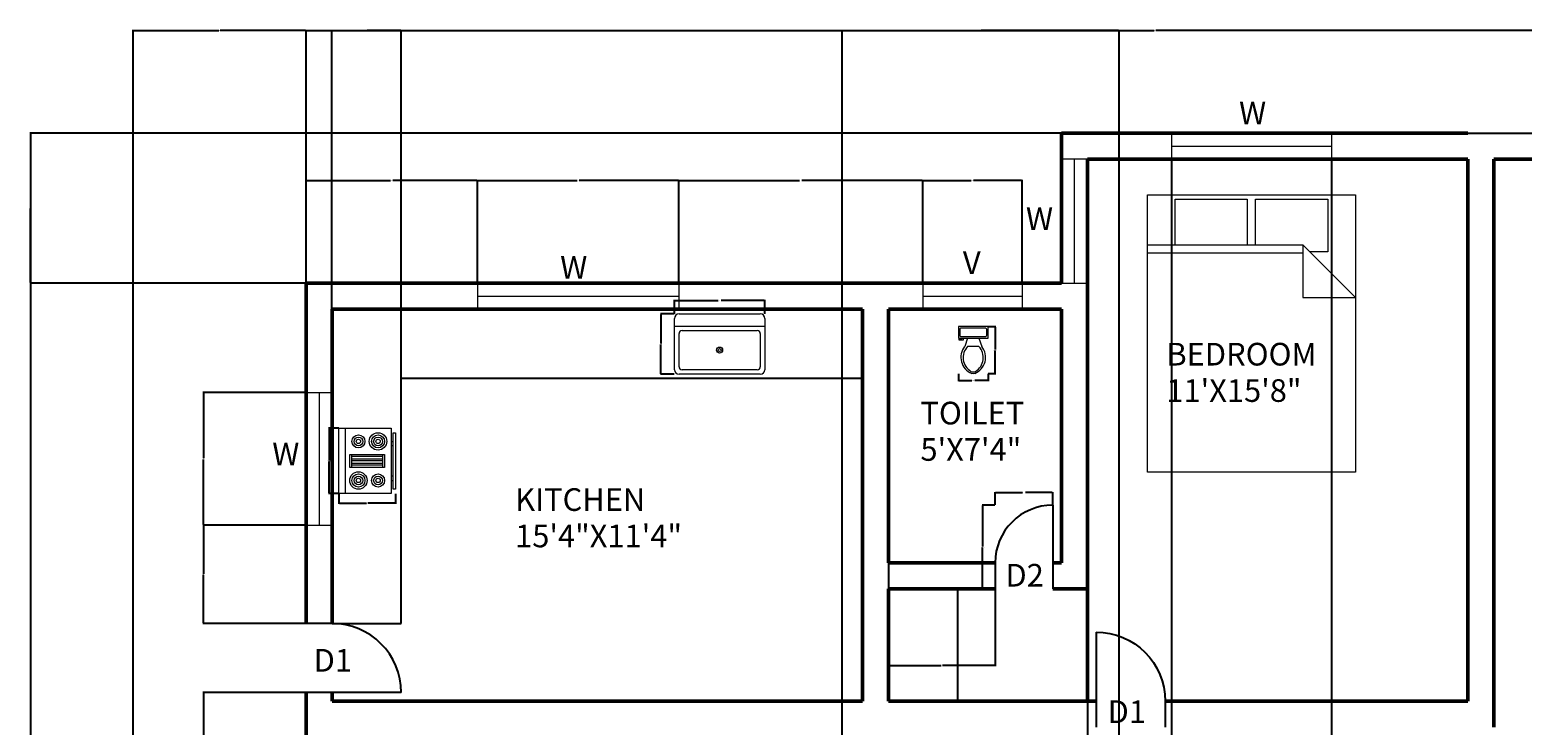
# Model space of a CAD drawing. Units: feet. Extents: x 1544 to 2324, y 1847 to 2475.
# Tile 3 of 4: x 1544 to 2061, y 2234 to 2475. Entities that reach past the tile are written whole.
import ezdxf

# ---------------------------------------------------------------- set-up
doc = ezdxf.new("R2010")
doc.units = ezdxf.units.FT
for name, color, linetype, lineweight in [('A-ANNO-DIMS', 2, 'Continuous', 18), ('A-ANNO-TEXT', 7, 'Continuous', 18), ('A-AREA-IDEN', 7, 'Continuous', 20), ('A-DOOR', 4, 'Continuous', 25), ('A-EQPM', 8, 'Continuous', 18), ('A-FLOR-CASE', 8, 'Continuous', 25), ('A-FLOR-FIXT', 9, 'Continuous', 18), ('A-FURN', 8, 'Continuous', 18), ('A-GLAZ', 4, 'Continuous', 18), ('A-WALL', 7, 'Continuous', 50), ('C-PROP', 3, 'Continuous', 25)]:
    doc.layers.add(name, color=color, linetype=linetype, lineweight=lineweight)
doc.styles.get("Standard").update_dxf_attribs({"font": 'arial.ttf'})
doc.dimstyles.get("Standard").update_dxf_attribs({"dimtxt": 0.18, "dimasz": 0.18, "dimexe": 0.18, "dimexo": 0.0625, "dimgap": 0.09, "dimtad": 0, "dimtih": 1, "dimtoh": 1, "dimdec": 4, "dimzin": 0, "dimdsep": 46, "dimtxsty": 'Standard', "dimcen": 0.09, "dimadec": 0, "dimazin": 0, "dimtfac": 1, "dimtdec": 4, "dimtofl": 0, "dimtmove": 0, "dimatfit": 3, "dimfxl": 1, "dimtolj": 1, "dimtzin": 0, "dimarcsym": 0})

# ---------------------------------------------------------------- blocks, each defined once
blk = doc.blocks.new('Sink-single - 30 in top')
blk.add_line((-15, -3.999996), (15, -3.999996))
for points in [[(-13.5, 0), (13.5, 0)], [(-15, -18.499996), (-15, -1.5)], [(15, -1.5), (15, -18.499996)], [(-13.5, -17.499996), (-13.5, -6.499996)], [(-12.5, -5.499996), (12.5, -5.499996)], [(13.5, -6.499996), (13.5, -17.499996)], [(12.5, -18.499996), (-12.5, -18.499996)], [(13.5, -19.999996), (-13.5, -19.999996)]]:
    blk.add_lwpolyline(points)
for radius in [1, 0.5]:
    blk.add_circle((0, -11.999996), radius)
for centre, radius, start, end in [((-13.5, -1.5), 1.5, 90, 180), ((13.5, -1.5), 1.5, 0, 90), ((-12.5, -6.499996), 1, 90, 180), ((12.5, -6.499996), 1, 0, 90), ((-13.5, -18.499996), 1.5, 180, 270), ((-12.5, -17.499996), 1, 180, 270), ((12.5, -17.499996), 1, 270, 0), ((13.5, -18.499996), 1.5, 270, 0)]:
    blk.add_arc(centre, radius, start, end)
blk = doc.blocks.new('Range-Oven - 30 in top')
for p, q in [((0, -3), (30, -3)), ((12, -6), (18, -6)), ((13, -20), (13, -6)), ((14, -6), (14, -20)), ((15, -20), (15, -6)), ((16, -6), (16, -20)), ((17, -20), (17, -6)), ((18, -20), (12, -20)), ((6, -24), (6, -25)), ((8, -25), (8, -24)), ((22, -25), (22, -24)), ((24, -24), (24, -25))]:
    blk.add_line(p, q)
for points in [[(0, -24), (0, 0), (30, 0), (30, -24)], [(12, -21), (12, -5), (18, -5), (18, -21)], [(2, -26), (2, -25), (28, -25), (28, -26)]]:
    blk.add_lwpolyline(points, close=True)
for centre, radius in [((6, -9), 4), ((6, -9), 3), ((24, -9), 3), ((6, -9), 2), ((6, -9), 1), ((24, -9), 2), ((24, -9), 1), ((6, -18), 3), ((6, -18), 2), ((6, -18), 1), ((24, -18), 4), ((24, -18), 3), ((24, -18), 2), ((24, -18), 1)]:
    blk.add_circle(centre, radius)
blk = doc.blocks.new('Toilet - top')
for p, q in [((-10, -8.5), (-8, -8.5)), ((-10, -9.5), (-10, -8.5)), ((-7, -9.5), (-10, -9.5)), ((-8, -8.5), (-8, -8)), ((-7, -8), (-7, -9.5)), ((-4, -8), (-6, -14)), ((4, -8), (6, -14)), ((9.5, -6), (9.5, -2)), ((4, -14), (-4, -14))]:
    blk.add_line(p, q)
blk.add_lwpolyline([(10.5, -8), (10.5, 0), (-10.5, 0), (-10.5, -8)], close=True)
for points in [[(-9.5, -2), (-9.5, -6)], [(8.5, -1), (-8.5, -1)], [(-8.5, -7), (8.5, -7)]]:
    blk.add_lwpolyline(points)
for centre, radius, start, end in [((-8.6, -1.9), 0.884, 81.8699, 188.1301), ((-8.6, -6.1), 0.884, 171.8699, 278.1301), ((8.6, -1.9), 0.884, 351.8699, 98.1301), ((8.6, -6.1), 0.884, 261.8699, 8.1301), ((3.5, -21.6), 12.2, 141.4691, 247.9714), ((4.2, -21.8), 11.3, 136.3677, 238.9468), ((-3.5, -21.6), 12.2, 292.0284, 38.5307), ((-4.2, -21.8), 11.3, 301.053, 43.6321), ((0, -27.9), 4, 245.7318, 294.2682), ((0, -29), 4, 254.8605, 285.1395)]:
    blk.add_arc(centre, radius, start, end)
blk = doc.blocks.new('Bed - Queen')
for p, q in [((0, -80.00003), (0, 0)), ((0, 0), (59.99999, 0)), ((59.99999, 0), (59.99999, -80.00003)), ((7.99999, -1.2), (28.79998, -1.2)), ((7.99999, -14.4), (7.99999, -1.2)), ((28.79998, -1.2), (28.79998, -14.4)), ((31.19999, -1.2), (51.99999, -1.2)), ((31.19999, -14.4), (31.19999, -1.2)), ((51.99999, -1.2), (51.99999, -16.4)), ((0, -14.4), (44.8, -14.4)), ((44.8, -16.8), (0, -16.8)), ((59.99999, -29.6), (44.8, -14.4)), ((44.8, -14.4), (44.8, -29.6)), ((51.99999, -16.4), (46.79936, -16.4)), ((44.8, -29.6), (59.99999, -29.6)), ((59.99999, -80.00003), (0, -80.00003))]:
    blk.add_line(p, q)
blk = doc.blocks.new('DOOR-SINGLE-R24')
for p, q in [((9, 24), (0, 24)), ((33, 0), (0, 0))]:
    blk.add_line(p, q)
blk.add_arc((9, 0), 24, 0, 90)
blk = doc.blocks.new('DOOR-SINGLE-R20')
for p, q in [((20, 29), (20, 0)), ((0, 9), (0, 0))]:
    blk.add_line(p, q)
blk.add_arc((20, 9), 20, 90, 180)
blk = doc.blocks.new('*D13')
at = {"layer": 'A-ANNO-DIMS', "color": 0, "lineweight": -2, "transparency": 16777216}
for p, q in [((1878.49, 2310.67), (1874.02, 2310.67)), ((1874.2, 2310.49), (1874.2, 2296.35)), ((1874.2, 2281.85), (1874.2, 2295.99)), ((1878.49, 2281.67), (1874.02, 2281.67))]:
    blk.add_line(p, q, dxfattribs=at)
at = {"layer": 'A-ANNO-DIMS', "color": 0, "transparency": 16777216}
for points in [[(1874.17, 2310.49), (1874.23, 2310.49), (1874.2, 2310.67)], [(1874.17, 2281.85), (1874.23, 2281.85), (1874.2, 2281.67)]]:
    blk.add_solid(points, dxfattribs=at)
at = {"layer": 'Defpoints', "color": 0, "transparency": 16777216}
for p in [(1874.2, 2310.67), (1878.55, 2310.67), (1878.55, 2281.67)]:
    blk.add_point(p, dxfattribs=at)
at = {"layer": 'A-ANNO-DIMS', "color": 0, "transparency": 16777216, "insert": (1874.2, 2296.17), "char_height": 0.18, "attachment_point": 5}
blk.add_mtext('\\A1;D2 29 TYP.', dxfattribs=at)
blk = doc.blocks.new('*D14')
at = {"layer": 'A-ANNO-DIMS', "color": 0, "lineweight": -2, "transparency": 16777216}
for p, q in [((1878.55, 2310.73), (1878.55, 2315.2)), ((1878.73, 2315.02), (1888.02, 2315.02)), ((1898.37, 2315.02), (1889.08, 2315.02)), ((1898.55, 2310.73), (1898.55, 2315.2))]:
    blk.add_line(p, q, dxfattribs=at)
at = {"layer": 'A-ANNO-DIMS', "color": 0, "transparency": 16777216}
for points in [[(1878.73, 2315.05), (1878.73, 2314.99), (1878.55, 2315.02)], [(1898.37, 2315.05), (1898.37, 2314.99), (1898.55, 2315.02)]]:
    blk.add_solid(points, dxfattribs=at)
at = {"layer": 'Defpoints', "color": 0, "transparency": 16777216}
for p in [(1898.55, 2315.02), (1878.55, 2310.67), (1898.55, 2310.67)]:
    blk.add_point(p, dxfattribs=at)
at = {"layer": 'A-ANNO-DIMS', "color": 0, "transparency": 16777216, "insert": (1888.55, 2315.02), "char_height": 0.18, "attachment_point": 5}
blk.add_mtext('\\A1;20 TYP.', dxfattribs=at)
blk = doc.blocks.new('*D15')
at = {"layer": 'A-ANNO-DIMS', "color": 0, "lineweight": -2, "transparency": 16777216}
for p, q in [((1876.19, 2372.55), (1878.75, 2372.55)), ((1878.57, 2372.37), (1878.57, 2364.6)), ((1878.57, 2356.47), (1878.57, 2364.24)), ((1876.19, 2356.29), (1878.75, 2356.29))]:
    blk.add_line(p, q, dxfattribs=at)
at = {"layer": 'A-ANNO-DIMS', "color": 0, "transparency": 16777216}
for points in [[(1878.54, 2372.37), (1878.6, 2372.37), (1878.57, 2372.55)], [(1878.54, 2356.47), (1878.6, 2356.47), (1878.57, 2356.29)]]:
    blk.add_solid(points, dxfattribs=at)
at = {"layer": 'Defpoints', "color": 0, "transparency": 16777216}
for p in [(1876.13, 2372.55), (1878.57, 2372.55), (1876.13, 2356.29)]:
    blk.add_point(p, dxfattribs=at)
at = {"layer": 'A-ANNO-DIMS', "color": 0, "transparency": 16777216, "insert": (1878.57, 2364.42), "char_height": 0.18, "attachment_point": 5}
blk.add_mtext('\\A1;WC 16 TYP.', dxfattribs=at)
blk = doc.blocks.new('*D16')
at = {"layer": 'A-ANNO-DIMS', "color": 0, "lineweight": -2, "transparency": 16777216}
for p, q in [((1865.8, 2356.23), (1865.8, 2353.67)), ((1876.13, 2356.23), (1876.13, 2353.67)), ((1865.98, 2353.85), (1870.44, 2353.85)), ((1875.95, 2353.85), (1871.48, 2353.85))]:
    blk.add_line(p, q, dxfattribs=at)
at = {"layer": 'A-ANNO-DIMS', "color": 0, "transparency": 16777216}
for points in [[(1865.98, 2353.88), (1865.98, 2353.82), (1865.8, 2353.85)], [(1875.95, 2353.88), (1875.95, 2353.82), (1876.13, 2353.85)]]:
    blk.add_solid(points, dxfattribs=at)
at = {"layer": 'Defpoints', "color": 0, "transparency": 16777216}
for p in [(1865.8, 2356.29), (1876.13, 2356.29), (1876.13, 2353.85)]:
    blk.add_point(p, dxfattribs=at)
at = {"layer": 'A-ANNO-DIMS', "color": 0, "transparency": 16777216, "insert": (1870.96, 2353.85), "char_height": 0.18, "attachment_point": 5}
blk.add_mtext('\\A1;10 TYP.', dxfattribs=at)
blk = doc.blocks.new('*D21')
at = {"layer": 'A-ANNO-DIMS', "color": 0, "lineweight": -2, "transparency": 16777216}
for p, q in [((1767.34, 2377.02), (1767.34, 2381.83)), ((1767.52, 2381.65), (1782.48, 2381.65)), ((1798.49, 2381.65), (1783.54, 2381.65)), ((1798.67, 2377.02), (1798.67, 2381.83))]:
    blk.add_line(p, q, dxfattribs=at)
at = {"layer": 'A-ANNO-DIMS', "color": 0, "transparency": 16777216}
for points in [[(1767.52, 2381.68), (1767.52, 2381.62), (1767.34, 2381.65)], [(1798.49, 2381.68), (1798.49, 2381.62), (1798.67, 2381.65)]]:
    blk.add_solid(points, dxfattribs=at)
at = {"layer": 'Defpoints', "color": 0, "transparency": 16777216}
for p in [(1798.67, 2381.65), (1767.34, 2376.95), (1798.67, 2376.95)]:
    blk.add_point(p, dxfattribs=at)
at = {"layer": 'A-ANNO-DIMS', "color": 0, "transparency": 16777216, "insert": (1783.01, 2381.65), "char_height": 0.18, "attachment_point": 5}
blk.add_mtext('\\A1;SINK 31', dxfattribs=at)
blk = doc.blocks.new('*D22')
at = {"layer": 'A-ANNO-DIMS', "color": 0, "lineweight": -2, "transparency": 16777216}
for p, q in [((1767.28, 2376.95), (1762.46, 2376.95)), ((1762.64, 2376.77), (1762.64, 2366.69)), ((1762.64, 2356.25), (1762.64, 2366.33)), ((1767.28, 2356.07), (1762.46, 2356.07))]:
    blk.add_line(p, q, dxfattribs=at)
at = {"layer": 'A-ANNO-DIMS', "color": 0, "transparency": 16777216}
for points in [[(1762.61, 2376.77), (1762.67, 2376.77), (1762.64, 2376.95)], [(1762.61, 2356.25), (1762.67, 2356.25), (1762.64, 2356.07)]]:
    blk.add_solid(points, dxfattribs=at)
at = {"layer": 'Defpoints', "color": 0, "transparency": 16777216}
for p in [(1762.64, 2376.95), (1767.34, 2376.95), (1767.34, 2356.07)]:
    blk.add_point(p, dxfattribs=at)
at = {"layer": 'A-ANNO-DIMS', "color": 0, "transparency": 16777216, "insert": (1762.64, 2366.51), "char_height": 0.18, "attachment_point": 5}
blk.add_mtext('\\A1;21', dxfattribs=at)
blk = doc.blocks.new('*D23')
at = {"layer": 'A-ANNO-DIMS', "color": 0, "lineweight": -2, "transparency": 16777216}
for p, q in [((1650.88, 2337.3), (1647.37, 2337.3)), ((1647.55, 2337.12), (1647.55, 2326.18)), ((1647.55, 2314.88), (1647.55, 2325.82)), ((1650.88, 2314.7), (1647.37, 2314.7))]:
    blk.add_line(p, q, dxfattribs=at)
at = {"layer": 'A-ANNO-DIMS', "color": 0, "transparency": 16777216}
for points in [[(1647.52, 2337.12), (1647.58, 2337.12), (1647.55, 2337.3)], [(1647.52, 2314.88), (1647.58, 2314.88), (1647.55, 2314.7)]]:
    blk.add_solid(points, dxfattribs=at)
at = {"layer": 'Defpoints', "color": 0, "transparency": 16777216}
for p in [(1647.55, 2337.3), (1650.95, 2337.3), (1650.95, 2314.7)]:
    blk.add_point(p, dxfattribs=at)
at = {"layer": 'A-ANNO-DIMS', "color": 0, "transparency": 16777216, "insert": (1647.55, 2326), "char_height": 0.18, "attachment_point": 5}
blk.add_mtext('\\A1;RANGE 23', dxfattribs=at)
blk = doc.blocks.new('*D24')
at = {"layer": 'A-ANNO-DIMS', "color": 0, "lineweight": -2, "transparency": 16777216}
for p, q in [((1650.95, 2314.63), (1650.95, 2311.13)), ((1670.54, 2314.63), (1670.54, 2311.13)), ((1651.13, 2311.31), (1660.52, 2311.31)), ((1670.36, 2311.31), (1660.96, 2311.31))]:
    blk.add_line(p, q, dxfattribs=at)
at = {"layer": 'A-ANNO-DIMS', "color": 0, "transparency": 16777216}
for points in [[(1651.13, 2311.34), (1651.13, 2311.28), (1650.95, 2311.31)], [(1670.36, 2311.34), (1670.36, 2311.28), (1670.54, 2311.31)]]:
    blk.add_solid(points, dxfattribs=at)
at = {"layer": 'Defpoints', "color": 0, "transparency": 16777216}
for p in [(1650.95, 2314.7), (1670.54, 2314.7), (1650.95, 2311.31)]:
    blk.add_point(p, dxfattribs=at)
at = {"layer": 'A-ANNO-DIMS', "color": 0, "transparency": 16777216, "insert": (1660.74, 2311.31), "char_height": 0.18, "attachment_point": 5}
blk.add_mtext('\\A1;20', dxfattribs=at)
blk = doc.blocks.new('*D32')
at = {"layer": 'A-ANNO-DIMS', "color": 0, "lineweight": -2, "transparency": 16777216}
for p, q in [((1579.49, 2439.67), (1543.77, 2439.67)), ((1543.95, 2439.49), (1543.95, 2161.35)), ((1543.95, 1882.85), (1543.95, 2160.99)), ((1579.49, 1882.67), (1543.77, 1882.67))]:
    blk.add_line(p, q, dxfattribs=at)
at = {"layer": 'A-ANNO-DIMS', "color": 0, "transparency": 16777216}
for points in [[(1543.92, 2439.49), (1543.98, 2439.49), (1543.95, 2439.67)], [(1543.92, 1882.85), (1543.98, 1882.85), (1543.95, 1882.67)]]:
    blk.add_solid(points, dxfattribs=at)
at = {"layer": 'Defpoints', "color": 0, "transparency": 16777216}
for p in [(1543.95, 2439.67), (1579.55, 2439.67), (1579.55, 1882.67)]:
    blk.add_point(p, dxfattribs=at)
at = {"layer": 'A-ANNO-DIMS', "color": 0, "transparency": 16777216, "insert": (1543.95, 2161.17), "char_height": 0.18, "attachment_point": 5}
blk.add_mtext('\\A1;557', dxfattribs=at)
blk = doc.blocks.new('*D33')
at = {"layer": 'A-ANNO-DIMS', "color": 0, "lineweight": -2, "transparency": 16777216}
for p, q in [((1639.55, 2387.73), (1639.55, 2475.45)), ((1639.73, 2475.27), (1933.76, 2475.27)), ((2228.37, 2475.27), (1934.34, 2475.27)), ((2228.55, 2439.73), (2228.55, 2475.45))]:
    blk.add_line(p, q, dxfattribs=at)
at = {"layer": 'A-ANNO-DIMS', "color": 0, "transparency": 16777216}
for points in [[(1639.73, 2475.3), (1639.73, 2475.24), (1639.55, 2475.27)], [(2228.37, 2475.3), (2228.37, 2475.24), (2228.55, 2475.27)]]:
    blk.add_solid(points, dxfattribs=at)
at = {"layer": 'Defpoints', "color": 0, "transparency": 16777216}
for p in [(2228.55, 2475.27), (2228.55, 2439.67), (1639.55, 2387.67)]:
    blk.add_point(p, dxfattribs=at)
at = {"layer": 'A-ANNO-DIMS', "color": 0, "transparency": 16777216, "insert": (1934.05, 2475.27), "char_height": 0.18, "attachment_point": 5}
blk.add_mtext('\\A1;589', dxfattribs=at)
blk = doc.blocks.new('*D35')
at = {"layer": 'A-ANNO-DIMS', "color": 0, "lineweight": -2, "transparency": 16777216}
for p, q in [((1579.55, 2439.73), (1579.55, 2475.45)), ((1579.73, 2475.27), (1609.33, 2475.27)), ((1639.37, 2475.27), (1609.77, 2475.27)), ((1639.55, 2387.73), (1639.55, 2475.45))]:
    blk.add_line(p, q, dxfattribs=at)
at = {"layer": 'A-ANNO-DIMS', "color": 0, "transparency": 16777216}
for points in [[(1579.73, 2475.3), (1579.73, 2475.24), (1579.55, 2475.27)], [(1639.37, 2475.3), (1639.37, 2475.24), (1639.55, 2475.27)]]:
    blk.add_solid(points, dxfattribs=at)
at = {"layer": 'Defpoints', "color": 0, "transparency": 16777216}
for p in [(1639.55, 2475.27), (1579.55, 2439.67), (1639.55, 2387.67)]:
    blk.add_point(p, dxfattribs=at)
at = {"layer": 'A-ANNO-DIMS', "color": 0, "transparency": 16777216, "insert": (1609.55, 2475.27), "char_height": 0.18, "attachment_point": 5}
blk.add_mtext('\\A1;60', dxfattribs=at)
blk = doc.blocks.new('*D37')
at = {"layer": 'A-ANNO-DIMS', "color": 0, "lineweight": -2, "transparency": 16777216}
for p, q in [((1901.49, 2439.67), (1543.77, 2439.67)), ((1543.95, 2439.49), (1543.95, 2413.85)), ((1543.95, 2387.85), (1543.95, 2413.49)), ((1901.49, 2387.67), (1543.77, 2387.67))]:
    blk.add_line(p, q, dxfattribs=at)
at = {"layer": 'A-ANNO-DIMS', "color": 0, "transparency": 16777216}
for points in [[(1543.92, 2439.49), (1543.98, 2439.49), (1543.95, 2439.67)], [(1543.92, 2387.85), (1543.98, 2387.85), (1543.95, 2387.67)]]:
    blk.add_solid(points, dxfattribs=at)
at = {"layer": 'Defpoints', "color": 0, "transparency": 16777216}
for p in [(1543.95, 2439.67), (1901.55, 2439.67), (1901.55, 2387.67)]:
    blk.add_point(p, dxfattribs=at)
at = {"layer": 'A-ANNO-DIMS', "color": 0, "transparency": 16777216, "insert": (1543.95, 2413.67), "char_height": 0.18, "attachment_point": 5}
blk.add_mtext('\\A1;52', dxfattribs=at)
blk = doc.blocks.new('*D38')
at = {"layer": 'A-ANNO-DIMS', "color": 0, "lineweight": -2, "transparency": 16777216}
for p, q in [((1639.55, 2387.73), (1639.55, 2423.45)), ((1639.73, 2423.27), (1668.88, 2423.27)), ((1698.8, 2423.27), (1669.66, 2423.27)), ((1698.98, 2387.73), (1698.98, 2423.45))]:
    blk.add_line(p, q, dxfattribs=at)
at = {"layer": 'A-ANNO-DIMS', "color": 0, "transparency": 16777216}
for points in [[(1639.73, 2423.3), (1639.73, 2423.24), (1639.55, 2423.27)], [(1698.8, 2423.3), (1698.8, 2423.24), (1698.98, 2423.27)]]:
    blk.add_solid(points, dxfattribs=at)
at = {"layer": 'Defpoints', "color": 0, "transparency": 16777216}
for p in [(1698.98, 2423.27), (1639.55, 2387.67), (1698.98, 2387.67)]:
    blk.add_point(p, dxfattribs=at)
at = {"layer": 'A-ANNO-DIMS', "color": 0, "transparency": 16777216, "insert": (1669.27, 2423.27), "char_height": 0.18, "attachment_point": 5}
blk.add_mtext('\\A1;59.43', dxfattribs=at)
blk = doc.blocks.new('*D39')
at = {"layer": 'A-ANNO-DIMS', "color": 0, "lineweight": -2, "transparency": 16777216}
for p, q in [((1698.98, 2387.73), (1698.98, 2423.45)), ((1699.16, 2423.27), (1733.53, 2423.27)), ((1768.68, 2423.27), (1734.32, 2423.27)), ((1768.86, 2387.73), (1768.86, 2423.45))]:
    blk.add_line(p, q, dxfattribs=at)
at = {"layer": 'A-ANNO-DIMS', "color": 0, "transparency": 16777216}
for points in [[(1699.16, 2423.3), (1699.16, 2423.24), (1698.98, 2423.27)], [(1768.68, 2423.3), (1768.68, 2423.24), (1768.86, 2423.27)]]:
    blk.add_solid(points, dxfattribs=at)
at = {"layer": 'Defpoints', "color": 0, "transparency": 16777216}
for p in [(1768.86, 2423.27), (1698.98, 2387.67), (1768.86, 2387.67)]:
    blk.add_point(p, dxfattribs=at)
at = {"layer": 'A-ANNO-DIMS', "color": 0, "transparency": 16777216, "insert": (1733.92, 2423.27), "char_height": 0.18, "attachment_point": 5}
blk.add_mtext('\\A1;69.88', dxfattribs=at)
blk = doc.blocks.new('*D40')
at = {"layer": 'A-ANNO-DIMS', "color": 0, "lineweight": -2, "transparency": 16777216}
for p, q in [((1768.86, 2387.73), (1768.86, 2423.45)), ((1769.04, 2423.27), (1810.76, 2423.27)), ((1853.27, 2423.27), (1811.55, 2423.27)), ((1853.45, 2387.73), (1853.45, 2423.45))]:
    blk.add_line(p, q, dxfattribs=at)
at = {"layer": 'A-ANNO-DIMS', "color": 0, "transparency": 16777216}
for points in [[(1769.04, 2423.3), (1769.04, 2423.24), (1768.86, 2423.27)], [(1853.27, 2423.3), (1853.27, 2423.24), (1853.45, 2423.27)]]:
    blk.add_solid(points, dxfattribs=at)
at = {"layer": 'Defpoints', "color": 0, "transparency": 16777216}
for p in [(1853.45, 2423.27), (1768.86, 2387.67), (1853.45, 2387.67)]:
    blk.add_point(p, dxfattribs=at)
at = {"layer": 'A-ANNO-DIMS', "color": 0, "transparency": 16777216, "insert": (1811.16, 2423.27), "char_height": 0.18, "attachment_point": 5}
blk.add_mtext('\\A1;84.58', dxfattribs=at)
blk = doc.blocks.new('*D41')
at = {"layer": 'A-ANNO-DIMS', "color": 0, "lineweight": -2, "transparency": 16777216}
for p, q in [((1853.45, 2387.73), (1853.45, 2423.45)), ((1853.63, 2423.27), (1870.28, 2423.27)), ((1887.72, 2423.27), (1871.07, 2423.27)), ((1887.9, 2387.73), (1887.9, 2423.45))]:
    blk.add_line(p, q, dxfattribs=at)
at = {"layer": 'A-ANNO-DIMS', "color": 0, "transparency": 16777216}
for points in [[(1853.63, 2423.3), (1853.63, 2423.24), (1853.45, 2423.27)], [(1887.72, 2423.3), (1887.72, 2423.24), (1887.9, 2423.27)]]:
    blk.add_solid(points, dxfattribs=at)
at = {"layer": 'Defpoints', "color": 0, "transparency": 16777216}
for p in [(1887.9, 2423.27), (1853.45, 2387.67), (1887.9, 2387.67)]:
    blk.add_point(p, dxfattribs=at)
at = {"layer": 'A-ANNO-DIMS', "color": 0, "transparency": 16777216, "insert": (1870.67, 2423.27), "char_height": 0.18, "attachment_point": 5}
blk.add_mtext('\\A1;34.45', dxfattribs=at)
blk = doc.blocks.new('*D42')
at = {"layer": 'A-ANNO-DIMS', "color": 0, "lineweight": -2, "transparency": 16777216}
for p, q in [((1910.55, 2430.61), (1910.55, 1846.89)), ((1939.68, 2430.61), (1939.68, 1846.89)), ((1910.73, 1847.07), (1924.72, 1847.07)), ((1939.5, 1847.07), (1925.51, 1847.07))]:
    blk.add_line(p, q, dxfattribs=at)
at = {"layer": 'A-ANNO-DIMS', "color": 0, "transparency": 16777216}
for points in [[(1910.73, 1847.1), (1910.73, 1847.04), (1910.55, 1847.07)], [(1939.5, 1847.1), (1939.5, 1847.04), (1939.68, 1847.07)]]:
    blk.add_solid(points, dxfattribs=at)
at = {"layer": 'Defpoints', "color": 0, "transparency": 16777216}
for p in [(1910.55, 2430.67), (1939.68, 2430.67), (1939.68, 1847.07)]:
    blk.add_point(p, dxfattribs=at)
at = {"layer": 'A-ANNO-DIMS', "color": 0, "transparency": 16777216, "insert": (1925.12, 1847.07), "char_height": 0.18, "attachment_point": 5}
blk.add_mtext('\\A1;29.13', dxfattribs=at)
blk = doc.blocks.new('*D43')
at = {"layer": 'A-ANNO-DIMS', "color": 0, "lineweight": -2, "transparency": 16777216}
for p, q in [((1939.68, 2430.61), (1939.68, 1846.89)), ((1995.24, 2430.61), (1995.24, 1846.89)), ((1939.86, 1847.07), (1967.07, 1847.07)), ((1995.06, 1847.07), (1967.85, 1847.07))]:
    blk.add_line(p, q, dxfattribs=at)
at = {"layer": 'A-ANNO-DIMS', "color": 0, "transparency": 16777216}
for points in [[(1939.86, 1847.1), (1939.86, 1847.04), (1939.68, 1847.07)], [(1995.06, 1847.1), (1995.06, 1847.04), (1995.24, 1847.07)]]:
    blk.add_solid(points, dxfattribs=at)
at = {"layer": 'Defpoints', "color": 0, "transparency": 16777216}
for p in [(1939.68, 2430.67), (1995.24, 2430.67), (1995.24, 1847.07)]:
    blk.add_point(p, dxfattribs=at)
at = {"layer": 'A-ANNO-DIMS', "color": 0, "transparency": 16777216, "insert": (1967.46, 1847.07), "char_height": 0.18, "attachment_point": 5}
blk.add_mtext('\\A1;55.55', dxfattribs=at)
blk = doc.blocks.new('*D53')
at = {"layer": 'A-ANNO-DIMS', "color": 0, "lineweight": -2, "transparency": 16777216}
for p, q in [((1825.55, 2103.73), (1825.55, 2475.45)), ((1825.73, 2475.27), (1873.34, 2475.27)), ((1921.37, 2475.27), (1873.77, 2475.27)), ((1921.55, 2103.73), (1921.55, 2475.45))]:
    blk.add_line(p, q, dxfattribs=at)
at = {"layer": 'A-ANNO-DIMS', "color": 0, "transparency": 16777216}
for points in [[(1825.73, 2475.3), (1825.73, 2475.24), (1825.55, 2475.27)], [(1921.37, 2475.3), (1921.37, 2475.24), (1921.55, 2475.27)]]:
    blk.add_solid(points, dxfattribs=at)
at = {"layer": 'Defpoints', "color": 0, "transparency": 16777216}
for p in [(1921.55, 2475.27), (1825.55, 2103.67), (1921.55, 2103.67)]:
    blk.add_point(p, dxfattribs=at)
at = {"layer": 'A-ANNO-DIMS', "color": 0, "transparency": 16777216, "insert": (1873.55, 2475.27), "char_height": 0.18, "attachment_point": 5}
blk.add_mtext('\\A1;96', dxfattribs=at)
blk = doc.blocks.new('*D63')
at = {"layer": 'A-ANNO-DIMS', "color": 0, "lineweight": -2, "transparency": 16777216}
for p, q in [((1639.49, 2245.67), (1603.77, 2245.67)), ((1603.95, 2245.49), (1603.95, 2227.85)), ((1603.95, 2209.85), (1603.95, 2227.49)), ((1639.49, 2209.67), (1603.77, 2209.67))]:
    blk.add_line(p, q, dxfattribs=at)
at = {"layer": 'A-ANNO-DIMS', "color": 0, "transparency": 16777216}
for points in [[(1603.92, 2245.49), (1603.98, 2245.49), (1603.95, 2245.67)], [(1603.92, 2209.85), (1603.98, 2209.85), (1603.95, 2209.67)]]:
    blk.add_solid(points, dxfattribs=at)
at = {"layer": 'Defpoints', "color": 0, "transparency": 16777216}
for p in [(1603.95, 2245.67), (1639.55, 2245.67), (1639.55, 2209.67)]:
    blk.add_point(p, dxfattribs=at)
at = {"layer": 'A-ANNO-DIMS', "color": 0, "transparency": 16777216, "insert": (1603.95, 2227.67), "char_height": 0.18, "attachment_point": 5}
blk.add_mtext('\\A1;36', dxfattribs=at)
blk = doc.blocks.new('*D64')
at = {"layer": 'A-ANNO-DIMS', "color": 0, "lineweight": -2, "transparency": 16777216}
for p, q in [((1639.49, 2303.73), (1603.77, 2303.73)), ((1603.95, 2303.55), (1603.95, 2286.88)), ((1603.95, 2269.85), (1603.95, 2286.52)), ((1639.49, 2269.67), (1603.77, 2269.67))]:
    blk.add_line(p, q, dxfattribs=at)
at = {"layer": 'A-ANNO-DIMS', "color": 0, "transparency": 16777216}
for points in [[(1603.92, 2303.55), (1603.98, 2303.55), (1603.95, 2303.73)], [(1603.92, 2269.85), (1603.98, 2269.85), (1603.95, 2269.67)]]:
    blk.add_solid(points, dxfattribs=at)
at = {"layer": 'Defpoints', "color": 0, "transparency": 16777216}
for p in [(1603.95, 2303.73), (1639.55, 2303.73), (1639.55, 2269.67)]:
    blk.add_point(p, dxfattribs=at)
at = {"layer": 'A-ANNO-DIMS', "color": 0, "transparency": 16777216, "insert": (1603.95, 2286.7), "char_height": 0.18, "attachment_point": 5}
blk.add_mtext('\\A1;34.064', dxfattribs=at)
blk = doc.blocks.new('*D65')
at = {"layer": 'A-ANNO-DIMS', "color": 0, "lineweight": -2, "transparency": 16777216}
for p, q in [((1639.49, 2349.71), (1603.77, 2349.71)), ((1603.95, 2349.53), (1603.95, 2326.9)), ((1603.95, 2303.91), (1603.95, 2326.54)), ((1639.49, 2303.73), (1603.77, 2303.73))]:
    blk.add_line(p, q, dxfattribs=at)
at = {"layer": 'A-ANNO-DIMS', "color": 0, "transparency": 16777216}
for points in [[(1603.92, 2349.53), (1603.98, 2349.53), (1603.95, 2349.71)], [(1603.92, 2303.91), (1603.98, 2303.91), (1603.95, 2303.73)]]:
    blk.add_solid(points, dxfattribs=at)
at = {"layer": 'Defpoints', "color": 0, "transparency": 16777216}
for p in [(1603.95, 2349.71), (1639.55, 2349.71), (1639.55, 2303.73)]:
    blk.add_point(p, dxfattribs=at)
at = {"layer": 'A-ANNO-DIMS', "color": 0, "transparency": 16777216, "insert": (1603.95, 2326.72), "char_height": 0.18, "attachment_point": 5}
blk.add_mtext('\\A1;45.97', dxfattribs=at)
blk = doc.blocks.new('*D71')
at = {"layer": 'A-ANNO-DIMS', "color": 0, "lineweight": -2, "transparency": 16777216}
for p, q in [((1648.55, 2269.73), (1648.55, 2475.45)), ((1648.73, 2475.27), (1660.33, 2475.27)), ((1672.37, 2475.27), (1660.77, 2475.27)), ((1672.55, 2269.73), (1672.55, 2475.45))]:
    blk.add_line(p, q, dxfattribs=at)
at = {"layer": 'A-ANNO-DIMS', "color": 0, "transparency": 16777216}
for points in [[(1648.73, 2475.3), (1648.73, 2475.24), (1648.55, 2475.27)], [(1672.37, 2475.3), (1672.37, 2475.24), (1672.55, 2475.27)]]:
    blk.add_solid(points, dxfattribs=at)
at = {"layer": 'Defpoints', "color": 0, "transparency": 16777216}
for p in [(1648.55, 2475.27), (1648.55, 2269.67), (1672.55, 2269.67)]:
    blk.add_point(p, dxfattribs=at)
at = {"layer": 'A-ANNO-DIMS', "color": 0, "transparency": 16777216, "insert": (1660.55, 2475.27), "char_height": 0.18, "attachment_point": 5}
blk.add_mtext('\\A1;24', dxfattribs=at)
blk = doc.blocks.new('*D72')
at = {"layer": 'A-ANNO-DIMS', "color": 0, "lineweight": -2, "transparency": 16777216}
for p, q in [((1841.55, 2290.61), (1841.55, 2254.89)), ((1878.55, 2290.61), (1878.55, 2254.89)), ((1841.73, 2255.07), (1859.84, 2255.07)), ((1878.37, 2255.07), (1860.27, 2255.07))]:
    blk.add_line(p, q, dxfattribs=at)
at = {"layer": 'A-ANNO-DIMS', "color": 0, "transparency": 16777216}
for points in [[(1841.73, 2255.1), (1841.73, 2255.04), (1841.55, 2255.07)], [(1878.37, 2255.1), (1878.37, 2255.04), (1878.55, 2255.07)]]:
    blk.add_solid(points, dxfattribs=at)
at = {"layer": 'Defpoints', "color": 0, "transparency": 16777216}
for p in [(1841.55, 2290.67), (1878.55, 2290.67), (1841.55, 2255.07)]:
    blk.add_point(p, dxfattribs=at)
at = {"layer": 'A-ANNO-DIMS', "color": 0, "transparency": 16777216, "insert": (1860.05, 2255.07), "char_height": 0.18, "attachment_point": 5}
blk.add_mtext('\\A1;37', dxfattribs=at)

msp = doc.modelspace()

# ---------------------------------------------------------------- linework, layer by layer
at = {"layer": 'A-FLOR-CASE'}
for p, q in [((1672.5539, 2354.6692), (1832.5539, 2354.6692)), ((1672.5539, 2269.6692), (1672.5539, 2354.6692)), ((1865.5539, 2281.6692), (1865.5539, 2242.6692)), ((1648.5539, 2269.6692), (1672.5539, 2269.6692))]:
    msp.add_line(p, q, dxfattribs=at)
at = {"layer": 'A-GLAZ'}
for p, q in [((1939.6827, 2439.6692), (1939.6827, 2430.6692)), ((1995.2363, 2439.6692), (1995.2363, 2430.6692)), ((1939.6827, 2435.1692), (1995.2363, 2435.1692)), ((1910.5539, 2430.6692), (1901.5539, 2430.6692)), ((1906.0539, 2387.6692), (1906.0539, 2430.6692)), ((1698.9841, 2387.6692), (1698.9841, 2378.6692)), ((1768.8646, 2387.6692), (1768.8646, 2378.6692)), ((1853.4486, 2387.6692), (1853.4486, 2378.6692)), ((1887.8991, 2387.6692), (1887.8991, 2378.6692)), ((1901.5539, 2387.6692), (1910.5539, 2387.6692)), ((1698.9841, 2383.1692), (1768.8646, 2383.1692)), ((1853.4486, 2383.1692), (1887.8991, 2383.1692)), ((1639.5539, 2349.7058), (1648.5539, 2349.7058)), ((1644.0539, 2349.7058), (1644.0539, 2303.733)), ((1639.5539, 2303.733), (1648.5539, 2303.733))]:
    msp.add_line(p, q, dxfattribs=at)
at = {"layer": 'A-WALL'}
for p, q in [((1901.5539, 2439.6692), (1901.5539, 2387.6692)), ((2042.5539, 2439.6692), (1901.5539, 2439.6692)), ((2042.5539, 2430.6692), (1910.5539, 2430.6692)), ((1910.5539, 2430.6692), (1910.5539, 2378.2983)), ((2042.5539, 2242.6692), (2042.5539, 2430.6692)), ((2051.5539, 2233.6692), (2051.5539, 2430.6692)), ((2051.5539, 2430.6692), (2219.5539, 2430.6692)), ((1639.5539, 2387.6692), (1901.5539, 2387.6692)), ((1639.5539, 2269.6692), (1639.5539, 2387.6692)), ((1841.5539, 2387.6692), (1901.5539, 2387.6692)), ((1648.5539, 2378.6692), (1832.5539, 2378.6692)), ((1648.5539, 2269.6692), (1648.5539, 2378.6692)), ((1832.5539, 2378.6692), (1832.5539, 2242.6692)), ((1841.5539, 2378.6692), (1841.5539, 2290.6692)), ((1841.5539, 2378.6692), (1901.5539, 2378.6692)), ((1901.5539, 2378.6692), (1901.5539, 2290.6692)), ((1901.5539, 2378.6692), (1901.5539, 2378.2983)), ((1910.5539, 2378.6692), (1910.5539, 2242.6692)), ((1878.5539, 2290.6692), (1841.5539, 2290.6692)), ((1901.5539, 2290.6692), (1898.5539, 2290.6692)), ((1841.5539, 2281.6692), (1841.5539, 2242.6692)), ((1878.5539, 2281.6692), (1841.5539, 2281.6692)), ((1910.5539, 2281.6692), (1898.5539, 2281.6692)), ((1639.5539, 1942.6692), (1639.5539, 2245.6692)), ((1648.5539, 2242.6692), (1648.5539, 2245.6692)), ((1832.5539, 2242.6692), (1648.5539, 2242.6692)), ((1841.5539, 2242.6692), (1910.5539, 2242.6692)), ((1910.5539, 2242.6692), (1913.5539, 2242.6692)), ((1937.5539, 2242.6692), (2042.5539, 2242.6692))]:
    msp.add_line(p, q, dxfattribs=at)
at = {"layer": 'C-PROP'}
for p, q in [((1901.5539, 2439.6692), (1579.5539, 2439.6692)), ((1579.5539, 1882.6692), (1579.5539, 2439.6692)), ((1901.5539, 2439.6692), (2288.5539, 2439.6692))]:
    msp.add_line(p, q, dxfattribs=at)

# ---------------------------------------------------------------- block references
at = {"layer": 'A-DOOR'}
for name, p in [('DOOR-SINGLE-R20', (1878.554, 2281.669)), ('DOOR-SINGLE-R24', (1639.554, 2245.669))]:
    msp.add_blockref(name, p, dxfattribs=at)
at = {"layer": 'A-DOOR', "extrusion": (0, 0, -1), "zscale": -1, "rotation": 90.00000000000003}
msp.add_blockref('DOOR-SINGLE-R24', (-1913.5537, 2233.6693), dxfattribs=at)
at = {"layer": 'A-EQPM', "xscale": 0.7535025227486893, "yscale": 0.7535025227486893, "zscale": 0.7535025227486893, "rotation": 90}
msp.add_blockref('Range-Oven - 30 in top', (1650.9454, 2314.6971), dxfattribs=at)
at = {"layer": 'A-FLOR-FIXT'}
for name, p, xscale, yscale, zscale in [('Sink-single - 30 in top', (1783.0077, 2376.9528), 1.044357894417281, 1.044357894417281, 1.044357894417281), ('Toilet - top', (1870.9641, 2372.553), 0.4921201164889298, 0.4921201164889298, 0.4921201164889298)]:
    msp.add_blockref(name, p, dxfattribs=dict(at, xscale=xscale, yscale=yscale, zscale=zscale))
at = {"layer": 'A-FURN', "xscale": 1.20179462178574, "yscale": 1.20179462178574, "zscale": 1.20179462178574}
msp.add_blockref('Bed - Queen', (1931.4137, 2418.2367), dxfattribs=at)

# ---------------------------------------------------------------- texts
at = {"layer": 'A-ANNO-TEXT'}
for s, height, p in [('W', 7.8492, (1963.1598, 2442.7056)), ('W', 7.8492, (1889.25, 2406.0308)), ('W', 7.8492, (1727.6998, 2389.1538)), ('V', 7.8492, (1867.3682, 2390.7666)), ('W', 7.8492, (1627.8282, 2324.5076)), ('D2', 7.84917, (1882.1412, 2282.4398)), ('D1', 7.84917, (1642.1692, 2252.9465)), ('D1', 7.84917, (1917.5541, 2235.1257))]:
    msp.add_text(s, height=height, dxfattribs=at).set_placement(p)
at = {"layer": 'A-AREA-IDEN'}
for s, height, p in [('BEDROOM', 7.84917, (1937.9498, 2359.0829)), ('11\'X15\'8"', 7.84917, (1937.9498, 2346.4739)), ('TOILET', 7.84917, (1852.649, 2338.6623)), ('5\'X7\'4"', 7.84917, (1852.649, 2326.0533)), ('KITCHEN', 7.84917, (1712.0631, 2308.6745)), ('15\'4"X11\'4"', 7.849169, (1712.0631, 2296.0655))]:
    msp.add_text(s, height=height, dxfattribs=at).set_placement(p)

# ---------------------------------------------------------------- dimensions: what is measured, and where the dimension line sits
at = {"layer": 'A-ANNO-DIMS'}
for base, p1, p2, override, picture, middle in [((1639.5539, 2475.2692), (1579.5539, 2439.6692), (1639.5539, 2387.6692), {"dimdec": 0, "dimlfac": 1, "dimrnd": 0, "dimzin": 0, "dimdsep": 46, "dimlunit": 2}, '*D35', (1609.5539, 2475.2692)), ((2228.5539, 2475.2692), (1639.5539, 2387.6692), (2228.5539, 2439.6692), {"dimdec": 0, "dimlfac": 1, "dimrnd": 0, "dimzin": 0, "dimdsep": 46, "dimlunit": 2}, '*D33', (1934.0539, 2475.2692)), ((1648.5539, 2475.2692), (1672.5539, 2269.6692), (1648.5539, 2269.6692), {"dimdec": 0, "dimlfac": 1, "dimrnd": 0, "dimzin": 0, "dimdsep": 46, "dimlunit": 2}, '*D71', (1660.5539, 2475.2692)), ((1921.5539, 2475.2692), (1825.5539, 2103.6692), (1921.5539, 2103.6692), {"dimdec": 0, "dimlfac": 1, "dimrnd": 0, "dimzin": 0, "dimdsep": 46, "dimlunit": 2}, '*D53', (1873.5539, 2475.2692)), ((1939.6827, 1847.0692), (1910.5539, 2430.6692), (1939.6827, 2430.6692), {"dimdec": 2, "dimlfac": 1, "dimrnd": 0, "dimzin": 0, "dimdsep": 46, "dimlunit": 2}, '*D42', (1925.1183, 1847.0692)), ((1995.2363, 1847.0692), (1939.6827, 2430.6692), (1995.2363, 2430.6692), {"dimdec": 2, "dimlfac": 1, "dimrnd": 0, "dimzin": 0, "dimdsep": 46, "dimlunit": 2}, '*D43', (1967.4595, 1847.0692)), ((1698.9841, 2423.2692), (1639.5539, 2387.6692), (1698.9841, 2387.6692), {"dimdec": 2, "dimlfac": 1, "dimrnd": 0, "dimzin": 0, "dimdsep": 46, "dimlunit": 2}, '*D38', (1669.269, 2423.2692)), ((1768.8646, 2423.2692), (1698.9841, 2387.6692), (1768.8646, 2387.6692), {"dimdec": 2, "dimlfac": 1, "dimrnd": 0, "dimzin": 0, "dimdsep": 46, "dimlunit": 2}, '*D39', (1733.9244, 2423.2692)), ((1853.4486, 2423.2692), (1768.8646, 2387.6692), (1853.4486, 2387.6692), {"dimdec": 2, "dimlfac": 1, "dimrnd": 0, "dimzin": 0, "dimdsep": 46, "dimlunit": 2}, '*D40', (1811.1566, 2423.2692)), ((1887.8991, 2423.2692), (1853.4486, 2387.6692), (1887.8991, 2387.6692), {"dimdec": 2, "dimlfac": 1, "dimrnd": 0, "dimzin": 0, "dimdsep": 46, "dimlunit": 2}, '*D41', (1870.6738, 2423.2692))]:
    dim = msp.add_linear_dim(base=base, p1=p1, p2=p2, dimstyle='Standard', override=override, dxfattribs=at)
    dim.commit()
    dim.dimension.update_dxf_attribs({"geometry": picture, "text_midpoint": middle})
for base, p1, p2, angle, override, picture, middle in [((1543.9539, 2439.6692), (1579.5539, 1882.6692), (1579.5539, 2439.6692), 90, {"dimdec": 0, "dimlfac": 1, "dimrnd": 0, "dimzin": 0, "dimdsep": 46, "dimlunit": 2}, '*D32', (1543.9539, 2161.1692)), ((1543.9539, 2439.6692), (1901.5539, 2387.6692), (1901.5539, 2439.6692), 90, {"dimdec": 0, "dimlfac": 1, "dimrnd": 0, "dimzin": 0, "dimdsep": 46, "dimlunit": 2}, '*D37', (1543.9539, 2413.6692)), ((1762.6427, 2376.9528), (1767.3424, 2356.0656), (1767.3424, 2376.9528), 90, {"dimdec": 0, "dimlfac": 1, "dimrnd": 0, "dimzin": 0, "dimdsep": 46, "dimlunit": 2}, '*D22', (1762.6427, 2366.5092)), ((1603.9539, 2349.7058), (1639.5539, 2303.733), (1639.5539, 2349.7058), 90, {"dimdec": 2, "dimlfac": 1, "dimrnd": 0, "dimzin": 0, "dimdsep": 46, "dimlunit": 2}, '*D65', (1603.9539, 2326.7194)), ((1650.9454, 2311.3063), (1670.5364, 2314.6971), (1650.9454, 2314.6971), 180, {"dimdec": 0, "dimlfac": 1, "dimrnd": 0, "dimzin": 0, "dimdsep": 46, "dimlunit": 2}, '*D24', (1660.7409, 2311.3063)), ((1603.9539, 2303.733), (1639.5539, 2269.6692), (1639.5539, 2303.733), 90, {"dimdec": 3, "dimlfac": 1, "dimrnd": 0, "dimzin": 0, "dimdsep": 46, "dimlunit": 2}, '*D64', (1603.9539, 2286.7011)), ((1841.5539, 2255.0692), (1878.5539, 2290.6692), (1841.5539, 2290.6692), 180, {"dimdec": 0, "dimlfac": 1, "dimrnd": 0, "dimzin": 0, "dimdsep": 46, "dimlunit": 2}, '*D72', (1860.0539, 2255.0692)), ((1603.9539, 2245.6692), (1639.5539, 2209.6692), (1639.5539, 2245.6692), 90, {"dimdec": 0, "dimlfac": 1, "dimrnd": 0, "dimzin": 0, "dimdsep": 46, "dimlunit": 2}, '*D63', (1603.9539, 2227.6692))]:
    dim = msp.add_linear_dim(base=base, p1=p1, p2=p2, angle=angle, dimstyle='Standard', override=override, dxfattribs=at)
    dim.commit()
    dim.dimension.update_dxf_attribs({"geometry": picture, "text_midpoint": middle})
for base, p1, p2, text, picture, middle in [((1798.6731, 2381.6524), (1767.3424, 2376.9528), (1798.6731, 2376.9528), 'SINK <>', '*D21', (1783.0077, 2381.6524)), ((1876.1314, 2353.8509), (1865.7969, 2356.2903), (1876.1314, 2356.2903), '<> TYP.', '*D16', (1870.9641, 2353.8509)), ((1898.5539, 2315.0192), (1878.5539, 2310.6692), (1898.5539, 2310.6692), '<> TYP.', '*D14', (1888.5539, 2315.0192))]:
    dim = msp.add_linear_dim(base=base, p1=p1, p2=p2, text=text, dimstyle='Standard', override={"dimdec": 0, "dimlfac": 1, "dimrnd": 0, "dimzin": 0, "dimdsep": 46, "dimlunit": 2}, dxfattribs=at)
    dim.commit()
    dim.dimension.update_dxf_attribs({"geometry": picture, "text_midpoint": middle})
for base, p1, p2, text, picture, middle in [((1878.5708, 2372.553), (1876.1314, 2356.2903), (1876.1314, 2372.553), 'WC <> TYP.', '*D15', (1878.5708, 2364.4217)), ((1647.5546, 2337.3021), (1650.9454, 2314.6971), (1650.9454, 2337.3021), 'RANGE <>', '*D23', (1647.5546, 2325.9996)), ((1874.2039, 2310.6692), (1878.5539, 2281.6692), (1878.5539, 2310.6692), 'D2 <> TYP.', '*D13', (1874.2039, 2296.1692))]:
    dim = msp.add_linear_dim(base=base, p1=p1, p2=p2, angle=90, text=text, dimstyle='Standard', override={"dimdec": 0, "dimlfac": 1, "dimrnd": 0, "dimzin": 0, "dimdsep": 46, "dimlunit": 2}, dxfattribs=at)
    dim.commit()
    dim.dimension.update_dxf_attribs({"geometry": picture, "text_midpoint": middle})

doc.saveas('drawing.dxf')
